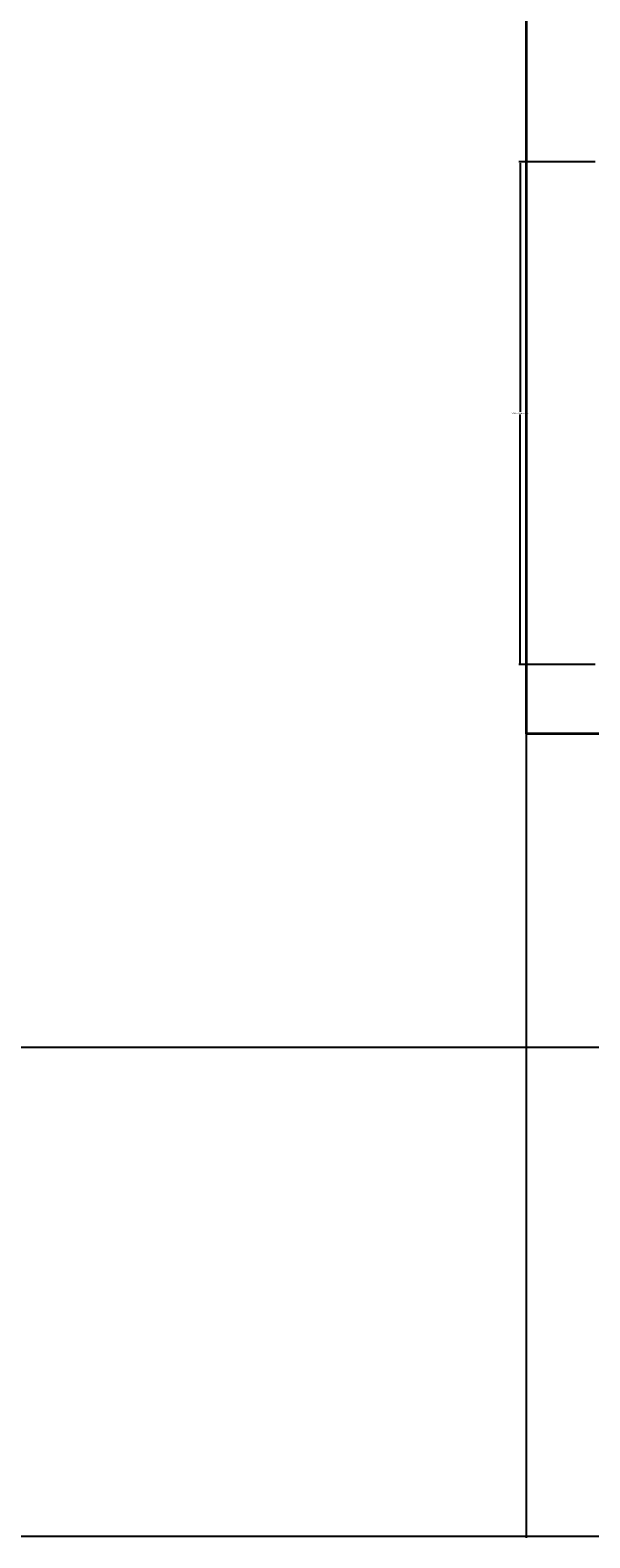
# Model space of a CAD drawing. Units: millimetres. Extents: x 27017497 to 27018854, y 7058029 to 7059154.
# Tile 62 of 91: x 27018246 to 27018319, y 7058029 to 7058224. Entities that reach past the tile are written whole.
import ezdxf

# ---------------------------------------------------------------- set-up
doc = ezdxf.new("R2010")
doc.units = ezdxf.units.MM
doc.layers.add('A-ANNO-DIMS', color=2, linetype='Continuous', lineweight=18)
doc.layers.add('A-WALL', color=7, linetype='Continuous', lineweight=35)
doc.styles.get("Standard").update_dxf_attribs({"font": 'arial.ttf'})
doc.dimstyles.get("Standard").update_dxf_attribs({"dimtxt": 0.18, "dimasz": 0.18, "dimexe": 0.18, "dimexo": 0.0625, "dimgap": 0.09, "dimtad": 0, "dimtih": 1, "dimtoh": 1, "dimdec": 4, "dimzin": 0, "dimdsep": 46, "dimtxsty": 'Standard', "dimcen": 0.09, "dimadec": 0, "dimazin": 0, "dimtfac": 1, "dimtdec": 4, "dimtofl": 0, "dimtmove": 0, "dimatfit": 3, "dimfxl": 1, "dimtolj": 1, "dimtzin": 0, "dimarcsym": 0})

# ---------------------------------------------------------------- blocks, each defined once
blk = doc.blocks.new('*D33')
at = {"layer": 'A-ANNO-DIMS', "color": 0, "lineweight": -2, "transparency": 16777216}
for p, q in [((27018319.54, 7058207.1), (27018309.64, 7058207.1)), ((27018309.82, 7058206.92), (27018309.82, 7058174.68)), ((27018309.82, 7058142.07), (27018309.82, 7058174.31)), ((27018319.54, 7058141.89), (27018309.64, 7058141.89))]:
    blk.add_line(p, q, dxfattribs=at)
at = {"layer": 'A-ANNO-DIMS', "color": 0, "transparency": 16777216}
for points in [[(27018309.79, 7058206.92), (27018309.85, 7058206.92), (27018309.82, 7058207.1)], [(27018309.79, 7058142.07), (27018309.85, 7058142.07), (27018309.82, 7058141.89)]]:
    blk.add_solid(points, dxfattribs=at)
at = {"layer": 'Defpoints', "color": 0, "transparency": 16777216}
for p in [(27018319.61, 7058207.1), (27018309.82, 7058141.89), (27018319.61, 7058141.89)]:
    blk.add_point(p, dxfattribs=at)
at = {"layer": 'A-ANNO-DIMS', "color": 0, "transparency": 16777216, "insert": (27018309.82, 7058174.49), "char_height": 0.18, "attachment_point": 5}
blk.add_mtext('\\A1;WARDROBE 65 TYP.', dxfattribs=at)
blk = doc.blocks.new('*D47')
at = {"layer": 'A-ANNO-DIMS', "color": 0, "lineweight": -2, "transparency": 16777216}
for p, q in [((27017561.17, 7058294.35), (27017561.17, 7058028.6)), ((27018790.61, 7058294.35), (27018790.61, 7058028.6)), ((27017561.35, 7058028.78), (27018175.43, 7058028.78)), ((27018790.43, 7058028.78), (27018176.34, 7058028.78))]:
    blk.add_line(p, q, dxfattribs=at)
at = {"layer": 'A-ANNO-DIMS', "color": 0, "transparency": 16777216}
for points in [[(27017561.35, 7058028.81), (27017561.35, 7058028.75), (27017561.17, 7058028.78)], [(27018790.43, 7058028.81), (27018790.43, 7058028.75), (27018790.61, 7058028.78)]]:
    blk.add_solid(points, dxfattribs=at)
at = {"layer": 'Defpoints', "color": 0, "transparency": 16777216}
for p in [(27017561.17, 7058294.41), (27018790.61, 7058294.41), (27018790.61, 7058028.78)]:
    blk.add_point(p, dxfattribs=at)
at = {"layer": 'A-ANNO-DIMS', "color": 0, "transparency": 16777216, "insert": (27018175.89, 7058028.78), "char_height": 0.18, "attachment_point": 5}
blk.add_mtext('\\A1;1229.4', dxfattribs=at)
blk = doc.blocks.new('*D48')
at = {"layer": 'A-ANNO-DIMS', "color": 0, "lineweight": -2, "transparency": 16777216}
for p, q in [((27018463.5, 7058622.91), (27017497.54, 7058622.91)), ((27017497.72, 7058622.73), (27017497.72, 7058357.75)), ((27017497.72, 7058092.41), (27017497.72, 7058357.39)), ((27018555.13, 7058092.23), (27017497.54, 7058092.23))]:
    blk.add_line(p, q, dxfattribs=at)
at = {"layer": 'A-ANNO-DIMS', "color": 0, "transparency": 16777216}
for points in [[(27017497.69, 7058622.73), (27017497.75, 7058622.73), (27017497.72, 7058622.91)], [(27017497.69, 7058092.41), (27017497.75, 7058092.41), (27017497.72, 7058092.23)]]:
    blk.add_solid(points, dxfattribs=at)
at = {"layer": 'Defpoints', "color": 0, "transparency": 16777216}
for p in [(27018463.56, 7058622.91), (27017497.72, 7058092.23), (27018555.19, 7058092.23)]:
    blk.add_point(p, dxfattribs=at)
at = {"layer": 'A-ANNO-DIMS', "color": 0, "transparency": 16777216, "insert": (27017497.72, 7058357.57), "char_height": 0.18, "attachment_point": 5}
blk.add_mtext('\\A1;530.7', dxfattribs=at)
blk = doc.blocks.new('*D51')
at = {"layer": 'A-ANNO-DIMS', "color": 0, "lineweight": -2, "transparency": 16777216}
for p, q in [((27018041.17, 7058345.35), (27018041.17, 7058028.6)), ((27018310.61, 7058345.35), (27018310.61, 7058028.6)), ((27018041.35, 7058028.78), (27018175.42, 7058028.78)), ((27018310.43, 7058028.78), (27018176.35, 7058028.78))]:
    blk.add_line(p, q, dxfattribs=at)
at = {"layer": 'A-ANNO-DIMS', "color": 0, "transparency": 16777216}
for points in [[(27018041.35, 7058028.81), (27018041.35, 7058028.75), (27018041.17, 7058028.78)], [(27018310.43, 7058028.81), (27018310.43, 7058028.75), (27018310.61, 7058028.78)]]:
    blk.add_solid(points, dxfattribs=at)
at = {"layer": 'Defpoints', "color": 0, "transparency": 16777216}
for p in [(27018041.17, 7058345.41), (27018310.61, 7058345.41), (27018310.61, 7058028.78)]:
    blk.add_point(p, dxfattribs=at)
at = {"layer": 'A-ANNO-DIMS', "color": 0, "transparency": 16777216, "insert": (27018175.89, 7058028.78), "char_height": 0.18, "attachment_point": 5}
blk.add_mtext('\\A1;269.44', dxfattribs=at)

msp = doc.modelspace()

# ---------------------------------------------------------------- linework, layer by layer
at = {"layer": 'A-WALL'}
for p, q in [((27018310.606, 7058589.912), (27018310.606, 7058169.223)), ((27018310.606, 7058386.357), (27018310.606, 7058132.912)), ((27018468.106, 7058132.912), (27018310.606, 7058132.912))]:
    msp.add_line(p, q, dxfattribs=at)

# ---------------------------------------------------------------- dimensions: what is measured, and where the dimension line sits
at = {"layer": 'A-ANNO-DIMS'}
dim = msp.add_linear_dim(base=(27017497.716, 7058092.23), p1=(27018463.561, 7058622.912), p2=(27018555.192, 7058092.23), angle=90, dimstyle='Standard', override={"dimdec": 1, "dimlfac": 1, "dimrnd": 0, "dimzin": 0, "dimdsep": 46, "dimlunit": 2}, dxfattribs=at)
dim.commit()
dim.dimension.update_dxf_attribs({"geometry": '*D48', "text_midpoint": (27017497.716, 7058357.571)})
for base, p1, p2, override, picture in [((27018310.606, 7058028.78), (27018041.166, 7058345.412), (27018310.606, 7058345.412), {"dimdec": 2, "dimlfac": 1, "dimrnd": 0, "dimzin": 0, "dimdsep": 46, "dimlunit": 2}, '*D51'), ((27018790.606, 7058028.78), (27017561.166, 7058294.412), (27018790.606, 7058294.412), {"dimdec": 1, "dimlfac": 1, "dimrnd": 0, "dimzin": 0, "dimdsep": 46, "dimlunit": 2}, '*D47')]:
    dim = msp.add_linear_dim(base=base, p1=p1, p2=p2, dimstyle='Standard', override=override, dxfattribs=at)
    dim.commit()
    dim.dimension.update_dxf_attribs({"geometry": picture, "text_midpoint": (27018175.886, 7058028.78)})
dim = msp.add_linear_dim(base=(27018309.824, 7058141.888), p1=(27018319.606, 7058207.1), p2=(27018319.606, 7058141.888), angle=270, text='WARDROBE <> TYP.', dimstyle='Standard', override={"dimdec": 0, "dimlfac": 1, "dimrnd": 0, "dimzin": 0, "dimdsep": 46, "dimlunit": 2}, dxfattribs=at)
dim.commit()
dim.dimension.update_dxf_attribs({"geometry": '*D33', "text_midpoint": (27018309.824, 7058174.494)})

doc.saveas('drawing.dxf')
